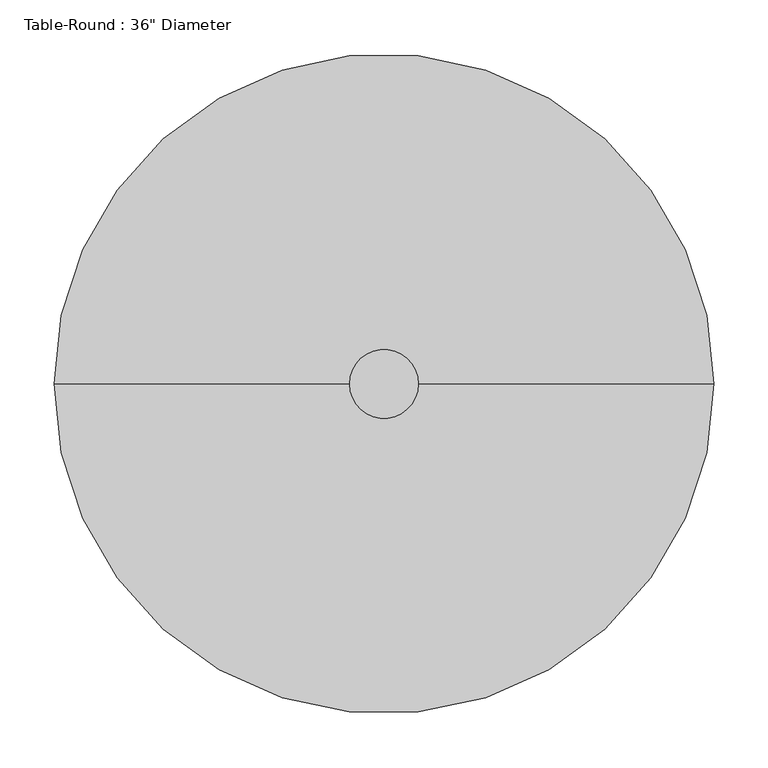
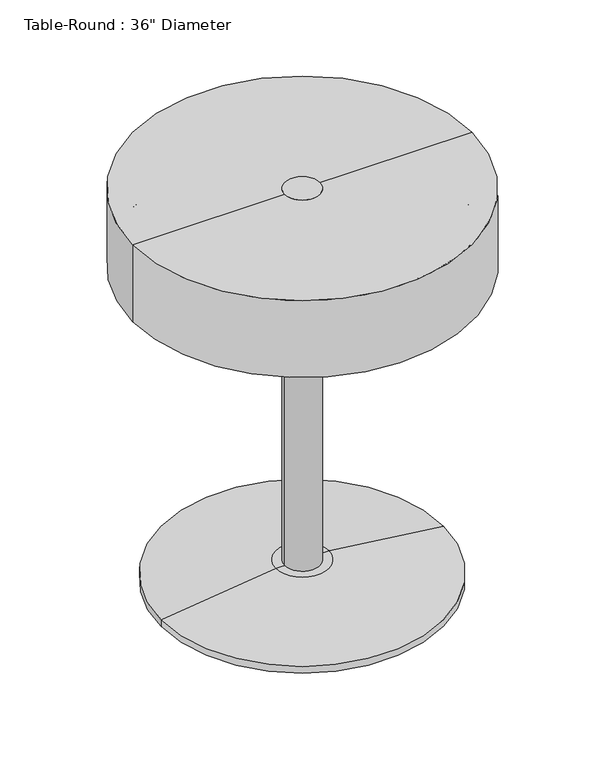
"""IFC4 building model written with IfcOpenShell, lengths in millimetres: furniture geometry."""

from ifc_helpers import new_model, si_unit, point, frame, origin, origin_2d, place, context, project, spatial, polyline, circle_curve, ellipse_curve, trimmed, segment, composite_curve, outline, extrude, source, transform, mapped, element, save
from ifc_brep_helpers import plane_surface, cylinder_surface, revolved_surface, advanced_brep


def furniture_3250926c(model_context):
    return source(origin(), model_context, "Body", "SolidModel", [
        extrude(outline(composite_curve([segment(trimmed(circle_curve(origin_2d(), 31.75), [point((-31.75, 0.0))], [point((31.75, 0.0))], False, "CARTESIAN"), True, "CONTINUOUS"), segment(trimmed(circle_curve(origin_2d(), 31.75), [point((31.75, 0.0))], [point((-31.75, 0.0))], False, "CARTESIAN"), True, "CONTINUOUS")], self_intersect=False)), frame((0.0, 0.0, 38.1), z_axis=(0.0, 0.0, 1.0), x_axis=(1.0, 0.0, 0.0)), (0.0, 0.0, 1.0), 704.85),
        advanced_brep(
        [(304.8, 0.0, 742.95), (-304.8, 0.0, 742.95), (0.0, 0.0, 742.95), (0.0, 0.0, 609.6), (-262.9011364, 0.0, 609.6), (262.9011364, 0.0, 609.6), (-299.5526659, 0.0, 603.1373465), (299.5526659, 0.0, 603.1373465), (-304.8, 0.0, 596.8838172), (304.8, 0.0, 596.8838172)],
        [
            (0, 1, circle_curve(frame((0.0, 0.0, 742.95), z_axis=(0.0, 0.0, 1.0), x_axis=(-1.0, 0.0, 0.0)), 304.8)),
            (1, 2),
            (2, 0),
            (1, 0, circle_curve(frame((0.0, 0.0, 742.95), z_axis=(0.0, 0.0, 1.0), x_axis=(-1.0, 0.0, 0.0)), 304.8)),
            (3, 4),
            (4, 5, circle_curve(frame((0.0, 0.0, 609.6), z_axis=(0.0, 0.0, -1.0), x_axis=(-1.0, 0.0, 0.0)), 262.9011364)),
            (5, 3),
            (5, 4, circle_curve(frame((0.0, 0.0, 609.6), z_axis=(0.0, 0.0, -1.0), x_axis=(-1.0, 0.0, 0.0)), 262.9011364)),
            (4, 6),
            (6, 7, circle_curve(frame((0.0, 0.0, 603.1373465), z_axis=(0.0, 0.0, -1.0), x_axis=(-1.0, 0.0, 0.0)), 299.5526659)),
            (7, 5),
            (7, 6, circle_curve(frame((0.0, 0.0, 603.1373465), z_axis=(0.0, 0.0, -1.0), x_axis=(-1.0, 0.0, 0.0)), 299.5526659)),
            (6, 8, circle_curve(frame((-298.45, 0.0, 596.8838172), z_axis=(0.0, -1.0, 0.0), x_axis=(1.0, 0.0, 0.0)), 6.35)),
            (8, 9, circle_curve(frame((0.0, 0.0, 596.8838172), z_axis=(0.0, 0.0, -1.0), x_axis=(-1.0, 0.0, 0.0)), 304.8)),
            (9, 7, circle_curve(frame((298.45, 0.0, 596.8838172), z_axis=(0.0, -1.0, 0.0), x_axis=(-1.0, 0.0, 0.0)), 6.35)),
            (9, 8, circle_curve(frame((0.0, 0.0, 596.8838172), z_axis=(0.0, 0.0, -1.0), x_axis=(-1.0, 0.0, 0.0)), 304.8)),
            (8, 1),
            (0, 9),
        ],
        [
            plane_surface(frame((0.0, 0.0, 742.95), z_axis=(0.0, 0.0, 1.0), x_axis=(-1.0, 0.0, 0.0))),
            plane_surface(frame((0.0, 0.0, 609.6), z_axis=(0.0, 0.0, -1.0), x_axis=(-1.0, 0.0, 0.0))),
            revolved_surface(polyline([(-299.5526659, 0.0, 603.1373465), (-262.9011364, 0.0, 609.6)]), (0.0, 0.0, 685.8), (0.0, 0.0, -1.0)),
            revolved_surface(trimmed(ellipse_curve(frame((-298.45, 0.0, 596.8838172), z_axis=(0.0, 1.0, 0.0), x_axis=(1.0, 0.0, 0.0)), 6.35, 6.35), [point((-304.8, 0.0, 596.8838172))], [point((-299.5526659, 0.0, 603.1373465))], True, "CARTESIAN"), (0.0, 0.0, 685.8), (0.0, 0.0, -1.0)),
            cylinder_surface(frame((0.0, 0.0, 685.8), z_axis=(0.0, 0.0, -1.0), x_axis=(-1.0, 0.0, 0.0)), 304.8),
        ],
        [
            (0, [[1, 2, 3]]),
            (0, [[4, -3, -2]]),
            (1, [[5, 6, 7]]),
            (1, [[-7, 8, -5]]),
            (2, [[-6, 9, 10, 11]]),
            (2, [[-8, -11, 12, -9]]),
            (3, [[-10, 13, 14, 15]]),
            (3, [[-12, -15, 16, -13]]),
            (4, [[-14, 17, -1, 18]]),
            (4, [[-16, -18, -4, -17]]),
        ],
    ),
        advanced_brep(
        [(0.0, 0.0, 0.0), (-254.0, 0.0, 0.0), (254.0, 0.0, 0.0), (47.625, 0.0, 38.1), (-47.625, 0.0, 38.1), (0.0, 0.0, 38.1), (254.0, 0.0, 12.7), (-254.0, 0.0, 12.7)],
        [
            (0, 1),
            (1, 2, circle_curve(frame((0.0, 0.0, 0.0), z_axis=(0.0, 0.0, -1.0), x_axis=(-1.0, 0.0, 0.0)), 254.0)),
            (2, 0),
            (2, 1, circle_curve(frame((0.0, 0.0, 0.0), z_axis=(0.0, 0.0, -1.0), x_axis=(-1.0, 0.0, 0.0)), 254.0)),
            (3, 4, circle_curve(frame((0.0, 0.0, 38.1), z_axis=(0.0, 0.0, 1.0), x_axis=(-1.0, 0.0, 0.0)), 47.625)),
            (4, 5),
            (5, 3),
            (4, 3, circle_curve(frame((0.0, 0.0, 38.1), z_axis=(0.0, 0.0, 1.0), x_axis=(-1.0, 0.0, 0.0)), 47.625)),
            (6, 7, circle_curve(frame((0.0, 0.0, 12.7), z_axis=(0.0, 0.0, 1.0), x_axis=(-1.0, 0.0, 0.0)), 254.0)),
            (7, 4),
            (3, 6),
            (7, 6, circle_curve(frame((0.0, 0.0, 12.7), z_axis=(0.0, 0.0, 1.0), x_axis=(-1.0, 0.0, 0.0)), 254.0)),
            (1, 7),
            (6, 2),
        ],
        [
            plane_surface(frame((0.0, 0.0, 0.0), z_axis=(0.0, 0.0, -1.0), x_axis=(-1.0, 0.0, 0.0))),
            plane_surface(frame((0.0, 0.0, 38.1), z_axis=(0.0, 0.0, 1.0), x_axis=(-1.0, 0.0, 0.0))),
            revolved_surface(polyline([(-47.625, 0.0, 38.1), (-254.0, 0.0, 12.7)]), (0.0, 0.0, 215.9), (0.0, 0.0, -1.0)),
            cylinder_surface(frame((0.0, 0.0, 215.9), z_axis=(0.0, 0.0, -1.0), x_axis=(-1.0, 0.0, 0.0)), 254.0),
        ],
        [
            (0, [[1, 2, 3]]),
            (0, [[-3, 4, -1]]),
            (1, [[5, 6, 7]]),
            (1, [[8, -7, -6]]),
            (2, [[9, 10, -5, 11]]),
            (2, [[12, -11, -8, -10]]),
            (3, [[-2, 13, -9, 14]]),
            (3, [[-4, -14, -12, -13]]),
        ],
    ),
    ])


if __name__ == "__main__":
    model = new_model("IFC4")
    model_context = context("Model", 3, world=origin())
    ifc_project = project(units=[si_unit("LENGTHUNIT", "METRE", prefix="MILLI")], contexts=[model_context])
    site = spatial("IfcSite", under=ifc_project)
    building = spatial("IfcBuilding", under=site)
    placement = place(None, origin())
    furniture_shape = furniture_3250926c(model_context)
    element("IfcFurniture", 1, ObjectType="Table-Round : 36\" Diameter", at=placement, inside=building, context=model_context, shape_type="MappedRepresentation", body=[
        mapped(furniture_shape, transform((0.0, 0.0, 0.0), x_axis=(1.0, 0.0, 0.0), y_axis=(0.0, 1.0, 0.0), z_axis=(0.0, 0.0, 1.0))),
    ])
    save(model, "model.ifc")

# Revit data of these elements
# Type "Table-Round : 36\" Diameter"
#   Assembly Code = "E2020200"
#   Base Radius = 0' - 10"
#   Height = 2' - 0"
#   Radius = 1' - 0"
#   Base Material = Steel, Chrome Plated
#   Top Material = Birch
#   Default Elevation = 0
# Element 1 (IfcFurniture, "Table-Round : 36\" Diameter")
#   Materials on its faces: "Steel, Chrome Plated", "Birch"
# Materials
#   "Steel, Chrome Plated": class "Metal", colour RGB 17 17 17, transparency 0, Description = "Chromiuim plated steel", Cost = 0
#   "Birch": class "Wood", colour RGB 224 178 126, transparency 0, Description = "Betula Alleghaniensis", Cost = 0
